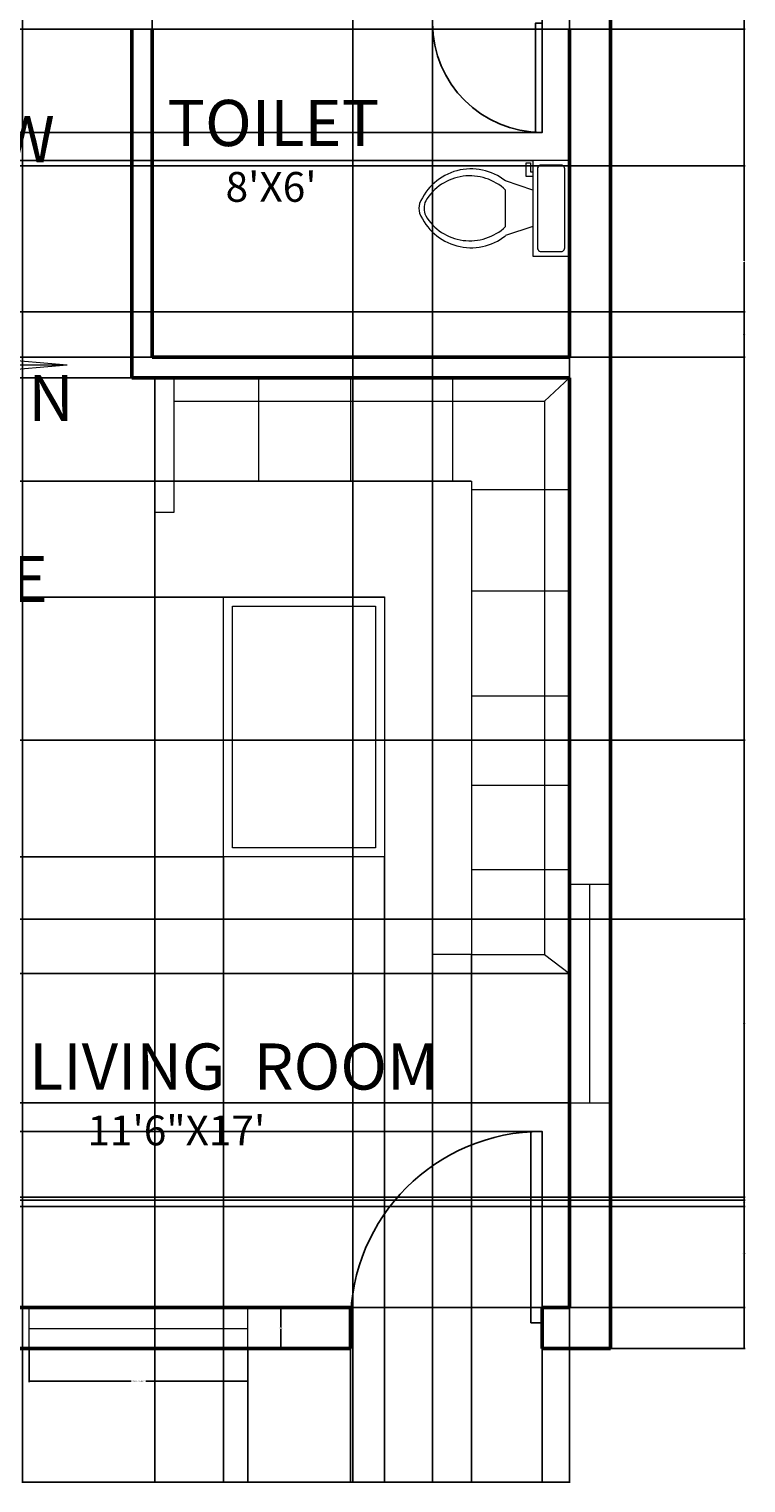
# Model space of a CAD drawing. Units: inches. Extents: x 19425 to 19848, y 45806 to 46417.
# Tile 4 of 5: x 19690 to 19848, y 45806 to 46125. Entities that reach past the tile are written whole.
import ezdxf

# ---------------------------------------------------------------- set-up
doc = ezdxf.new("R2010")
doc.units = ezdxf.units.IN
for name, color, linetype, lineweight in [('A-ANNO-DIMS', 2, 'Continuous', 18), ('A-ANNO-SYMB', 3, 'Continuous', 18), ('A-AREA-IDEN', 3, 'Continuous', 25), ('A-FLOR-FIXT', 2, 'Continuous', 20), ('door', 4, 'Continuous', 25), ('furniture', 2, 'Continuous', 18), ('wall', 6, 'Continuous', 50), ('window', 9, 'Continuous', 20)]:
    doc.layers.add(name, color=color, linetype=linetype, lineweight=lineweight)
doc.styles.get("Standard").update_dxf_attribs({"font": 'arial.ttf'})
doc.dimstyles.get("Standard").update_dxf_attribs({"dimtxt": 0.18, "dimasz": 0.18, "dimexe": 0.18, "dimexo": 0.0625, "dimgap": 0.09, "dimtad": 0, "dimtih": 1, "dimtoh": 1, "dimdec": 4, "dimzin": 0, "dimdsep": 46, "dimtxsty": 'Standard', "dimcen": 0.09, "dimadec": 0, "dimazin": 0, "dimtfac": 1, "dimtdec": 4, "dimtofl": 0, "dimtmove": 0, "dimatfit": 3, "dimfxl": 1, "dimtolj": 1, "dimtzin": 0, "dimarcsym": 0})

# ---------------------------------------------------------------- blocks, each defined once
blk = doc.blocks.new('*U2')
for p, q in [((0, 0), (0, -100)), ((750, 0), (750, -100))]:
    blk.add_line(p, q)
blk.add_lwpolyline([(0, 0), (0, 750), (43.75, 750), (43.75, 0)], close=True)
blk.add_arc((0, 0), 750, 0, 90)
blk = doc.blocks.new('Toilet - top')
for p, q in [((9.5, -6), (9.5, -2)), ((-10, -8.5), (-8, -8.5)), ((-10, -9.5), (-10, -8.5)), ((-7, -9.5), (-10, -9.5)), ((-8, -8.5), (-8, -8)), ((-7, -8), (-7, -9.5)), ((-4, -8), (-6, -14)), ((4, -8), (6, -14)), ((4, -14), (-4, -14))]:
    blk.add_line(p, q)
blk.add_lwpolyline([(10.5, -8), (10.5, 0), (-10.5, 0), (-10.5, -8)], close=True)
for points in [[(-9.5, -2), (-9.5, -6)], [(8.5, -1), (-8.5, -1)], [(-8.5, -7), (8.5, -7)]]:
    blk.add_lwpolyline(points)
for centre, radius, start, end in [((-8.62, -1.88), 0.884, 81.8699, 188.1301), ((8.62, -1.88), 0.884, 351.8699, 98.1301), ((-8.62, -6.12), 0.884, 171.8699, 278.1301), ((8.62, -6.12), 0.884, 261.8699, 8.1301), ((3.52, -21.58), 12.17, 141.4691, 247.9714), ((4.2, -21.82), 11.33, 136.3677, 238.9468), ((-3.52, -21.58), 12.17, 292.0284, 38.5307), ((-4.2, -21.82), 11.33, 301.053, 43.6321), ((0, -27.88), 4, 245.7318, 294.2682), ((0, -29), 4, 254.8605, 285.1395)]:
    blk.add_arc(centre, radius, start, end)
blk = doc.blocks.new('*U7')
at = {"layer": 'furniture'}
for p in [(-4.98, -28.71), (0, -23.73), (4.98, -28.71)]:
    blk.add_line(p, (0, 28.71), dxfattribs=at)
blk = doc.blocks.new('*U8')
at = {"layer": 'A-ANNO-SYMB', "transparency": 16777216}
blk.add_blockref('*U7', (19641.16, 46080.31), dxfattribs=at)
for p, rotation in [((19620.86, 46071.91), 45.00000000000001), ((19661.46, 46071.91), 315), ((19612.45, 46051.6), 90), ((19669.87, 46051.6), 270.0000000000001), ((19620.86, 46031.3), 135), ((19661.46, 46031.3), 225), ((19641.16, 46022.9), 180)]:
    blk.add_blockref('*U7', p, dxfattribs=dict(at, rotation=rotation))
blk = doc.blocks.new('WIN-48-CENTER-9')
for p, q in [((0, 48), (9, 48)), ((4.5, 0), (4.5, 48)), ((0, 0), (9, 0))]:
    blk.add_line(p, q)
blk = doc.blocks.new('WIN-48-OFFSET-9')
for p, q in [((0, 0), (0, 9)), ((48, 0), (48, 9)), ((48, 4.28), (0, 4.28))]:
    blk.add_line(p, q)
blk = doc.blocks.new('*D24')
at = {"layer": 'A-ANNO-DIMS', "color": 0, "lineweight": -2, "transparency": 16777216}
for p, q in [((19690.26, 45835.69), (19690.26, 45828.37)), ((19738.26, 45835.69), (19738.26, 45828.37)), ((19690.44, 45828.55), (19712.68, 45828.55)), ((19738.08, 45828.55), (19715.83, 45828.55))]:
    blk.add_line(p, q, dxfattribs=at)
at = {"layer": 'A-ANNO-DIMS', "color": 0, "transparency": 16777216}
for points in [[(19690.44, 45828.58), (19690.44, 45828.52), (19690.26, 45828.55)], [(19738.08, 45828.58), (19738.08, 45828.52), (19738.26, 45828.55)]]:
    blk.add_solid(points, dxfattribs=at)
at = {"layer": 'Defpoints', "color": 0, "transparency": 16777216}
for p in [(19690.26, 45835.75), (19738.26, 45835.75), (19738.26, 45828.55)]:
    blk.add_point(p, dxfattribs=at)
at = {"layer": 'A-ANNO-DIMS', "color": 0, "transparency": 16777216, "insert": (19714.26, 45828.55), "char_height": 0.18, "attachment_point": 5}
blk.add_mtext('\\A1;FRONT WINDOW 48 TYP.', dxfattribs=at)
blk = doc.blocks.new('*D25')
at = {"layer": 'A-ANNO-DIMS', "color": 0, "lineweight": -2, "transparency": 16777216}
for p, q in [((19738.32, 45844.75), (19745.64, 45844.75)), ((19745.46, 45844.57), (19745.46, 45840.44)), ((19745.46, 45835.93), (19745.46, 45840.07)), ((19738.32, 45835.75), (19745.64, 45835.75))]:
    blk.add_line(p, q, dxfattribs=at)
at = {"layer": 'A-ANNO-DIMS', "color": 0, "transparency": 16777216}
for points in [[(19745.43, 45844.57), (19745.49, 45844.57), (19745.46, 45844.75)], [(19745.43, 45835.93), (19745.49, 45835.93), (19745.46, 45835.75)]]:
    blk.add_solid(points, dxfattribs=at)
at = {"layer": 'Defpoints', "color": 0, "transparency": 16777216}
for p in [(19738.26, 45844.75), (19745.46, 45844.75), (19738.26, 45835.75)]:
    blk.add_point(p, dxfattribs=at)
at = {"layer": 'A-ANNO-DIMS', "color": 0, "transparency": 16777216, "insert": (19745.46, 45840.25), "char_height": 0.18, "attachment_point": 5}
blk.add_mtext('\\A1;9 TYP.', dxfattribs=at)
blk = doc.blocks.new('*D33')
at = {"layer": 'A-ANNO-DIMS', "color": 0, "lineweight": -2, "transparency": 16777216}
for p, q in [((19817.843662, 46312.754651), (19847.311162, 46312.754651)), ((19847.131162, 46312.574651), (19847.131162, 46074.434651)), ((19847.131162, 45835.934651), (19847.131162, 46074.074651)), ((19817.843662, 45835.754651), (19847.311162, 45835.754651))]:
    blk.add_line(p, q, dxfattribs=at)
at = {"layer": 'A-ANNO-DIMS', "color": 0, "transparency": 16777216}
for points in [[(19847.101162, 46312.574651), (19847.161162, 46312.574651), (19847.131162, 46312.754651)], [(19847.101162, 45835.934651), (19847.161162, 45835.934651), (19847.131162, 45835.754651)]]:
    blk.add_solid(points, dxfattribs=at)
at = {"layer": 'Defpoints', "color": 0, "transparency": 16777216}
for p in [(19817.781162, 46312.754651), (19847.131162, 46312.754651), (19817.781162, 45835.754651)]:
    blk.add_point(p, dxfattribs=at)
at = {"layer": 'A-ANNO-DIMS', "color": 0, "transparency": 16777216, "insert": (19847.131162, 46074.254651), "char_height": 0.18, "attachment_point": 5}
blk.add_mtext('\\A1;477', dxfattribs=at)
blk = doc.blocks.new('*D35')
at = {"layer": 'A-ANNO-DIMS', "color": 0, "lineweight": -2, "transparency": 16777216}
for p, q in [((19761.31, 46303.69), (19761.31, 45806.22)), ((19808.78, 46303.69), (19808.78, 45806.22)), ((19761.49, 45806.4), (19784.65, 45806.4)), ((19808.6, 45806.4), (19785.44, 45806.4))]:
    blk.add_line(p, q, dxfattribs=at)
at = {"layer": 'A-ANNO-DIMS', "color": 0, "transparency": 16777216}
for points in [[(19761.49, 45806.43), (19761.49, 45806.37), (19761.31, 45806.4)], [(19808.6, 45806.43), (19808.6, 45806.37), (19808.78, 45806.4)]]:
    blk.add_solid(points, dxfattribs=at)
at = {"layer": 'Defpoints', "color": 0, "transparency": 16777216}
for p in [(19761.31, 46303.75), (19808.78, 46303.75), (19808.78, 45806.4)]:
    blk.add_point(p, dxfattribs=at)
at = {"layer": 'A-ANNO-DIMS', "color": 0, "transparency": 16777216, "insert": (19785.04, 45806.4), "char_height": 0.18, "attachment_point": 5}
blk.add_mtext('\\A1;47.47', dxfattribs=at)
blk = doc.blocks.new('*D38')
at = {"layer": 'A-ANNO-DIMS', "color": 0, "lineweight": -2, "transparency": 16777216}
for p, q in [((19808.72, 45889.62), (19425.25, 45889.62)), ((19425.43, 45889.44), (19425.43, 45886.67)), ((19425.43, 45883.53), (19425.43, 45886.3)), ((19802.72, 45883.35), (19425.25, 45883.35))]:
    blk.add_line(p, q, dxfattribs=at)
at = {"layer": 'A-ANNO-DIMS', "color": 0, "transparency": 16777216}
for points in [[(19425.4, 45889.44), (19425.46, 45889.44), (19425.43, 45889.62)], [(19425.4, 45883.53), (19425.46, 45883.53), (19425.43, 45883.35)]]:
    blk.add_solid(points, dxfattribs=at)
at = {"layer": 'Defpoints', "color": 0, "transparency": 16777216}
for p in [(19425.43, 45889.62), (19808.78, 45889.62), (19802.78, 45883.35)]:
    blk.add_point(p, dxfattribs=at)
at = {"layer": 'A-ANNO-DIMS', "color": 0, "transparency": 16777216, "insert": (19425.43, 45886.49), "char_height": 0.18, "attachment_point": 5}
blk.add_mtext('\\A1;6.261', dxfattribs=at)
blk = doc.blocks.new('*D41')
at = {"layer": 'A-ANNO-DIMS', "color": 0, "lineweight": -2, "transparency": 16777216}
for p, q in [((19738.26, 45835.69), (19738.26, 45806.22)), ((19760.78, 45835.69), (19760.78, 45806.22)), ((19738.44, 45806.4), (19749.05, 45806.4)), ((19760.6, 45806.4), (19749.98, 45806.4))]:
    blk.add_line(p, q, dxfattribs=at)
at = {"layer": 'A-ANNO-DIMS', "color": 0, "transparency": 16777216}
for points in [[(19738.44, 45806.43), (19738.44, 45806.37), (19738.26, 45806.4)], [(19760.6, 45806.43), (19760.6, 45806.37), (19760.78, 45806.4)]]:
    blk.add_solid(points, dxfattribs=at)
at = {"layer": 'Defpoints', "color": 0, "transparency": 16777216}
for p in [(19738.26, 45835.75), (19760.78, 45835.75), (19760.78, 45806.4)]:
    blk.add_point(p, dxfattribs=at)
at = {"layer": 'A-ANNO-DIMS', "color": 0, "transparency": 16777216, "insert": (19749.52, 45806.4), "char_height": 0.18, "attachment_point": 5}
blk.add_mtext('\\A1;22.526', dxfattribs=at)
blk = doc.blocks.new('*D42')
at = {"layer": 'A-ANNO-DIMS', "color": 0, "lineweight": -2, "transparency": 16777216}
for p, q in [((19760.78, 45835.69), (19760.78, 45806.22)), ((19802.78, 45835.69), (19802.78, 45806.22)), ((19760.96, 45806.4), (19781.56, 45806.4)), ((19802.6, 45806.4), (19782, 45806.4))]:
    blk.add_line(p, q, dxfattribs=at)
at = {"layer": 'A-ANNO-DIMS', "color": 0, "transparency": 16777216}
for points in [[(19760.96, 45806.43), (19760.96, 45806.37), (19760.78, 45806.4)], [(19802.6, 45806.43), (19802.6, 45806.37), (19802.78, 45806.4)]]:
    blk.add_solid(points, dxfattribs=at)
at = {"layer": 'Defpoints', "color": 0, "transparency": 16777216}
for p in [(19760.78, 45835.75), (19802.78, 45835.75), (19802.78, 45806.4)]:
    blk.add_point(p, dxfattribs=at)
at = {"layer": 'A-ANNO-DIMS', "color": 0, "transparency": 16777216, "insert": (19781.78, 45806.4), "char_height": 0.18, "attachment_point": 5}
blk.add_mtext('\\A1;42', dxfattribs=at)
blk = doc.blocks.new('*D50')
at = {"layer": 'A-ANNO-DIMS', "color": 0, "lineweight": -2, "transparency": 16777216}
for p, q in [((19625.38, 45929.95), (19847.31, 45929.95)), ((19847.13, 45929.77), (19847.13, 45899.3)), ((19847.13, 45868.46), (19847.13, 45898.93)), ((19625.38, 45868.28), (19847.31, 45868.28))]:
    blk.add_line(p, q, dxfattribs=at)
at = {"layer": 'A-ANNO-DIMS', "color": 0, "transparency": 16777216}
for points in [[(19847.1, 45929.77), (19847.16, 45929.77), (19847.13, 45929.95)], [(19847.1, 45868.46), (19847.16, 45868.46), (19847.13, 45868.28)]]:
    blk.add_solid(points, dxfattribs=at)
at = {"layer": 'Defpoints', "color": 0, "transparency": 16777216}
for p in [(19625.31, 45929.95), (19847.13, 45929.95), (19625.31, 45868.28)]:
    blk.add_point(p, dxfattribs=at)
at = {"layer": 'A-ANNO-DIMS', "color": 0, "transparency": 16777216, "insert": (19847.13, 45899.11), "char_height": 0.18, "attachment_point": 5}
blk.add_mtext('\\A1;61.67', dxfattribs=at)
blk = doc.blocks.new('*D51')
at = {"layer": 'A-ANNO-DIMS', "color": 0, "lineweight": -2, "transparency": 16777216}
for p, q in [((19732.87, 45943.55), (19732.87, 45806.22)), ((19768.22, 45943.55), (19768.22, 45806.22)), ((19733.05, 45806.4), (19750.15, 45806.4)), ((19768.04, 45806.4), (19750.94, 45806.4))]:
    blk.add_line(p, q, dxfattribs=at)
at = {"layer": 'A-ANNO-DIMS', "color": 0, "transparency": 16777216}
for points in [[(19733.05, 45806.43), (19733.05, 45806.37), (19732.87, 45806.4)], [(19768.04, 45806.43), (19768.04, 45806.37), (19768.22, 45806.4)]]:
    blk.add_solid(points, dxfattribs=at)
at = {"layer": 'Defpoints', "color": 0, "transparency": 16777216}
for p in [(19732.87, 45943.61), (19768.22, 45943.61), (19768.22, 45806.4)]:
    blk.add_point(p, dxfattribs=at)
at = {"layer": 'A-ANNO-DIMS', "color": 0, "transparency": 16777216, "insert": (19750.55, 45806.4), "char_height": 0.18, "attachment_point": 5}
blk.add_mtext('\\A1;35.34', dxfattribs=at)
blk = doc.blocks.new('*D52')
at = {"layer": 'A-ANNO-DIMS', "color": 0, "lineweight": -2, "transparency": 16777216}
for p, q in [((19732.81, 46000.63), (19425.25, 46000.63)), ((19425.43, 46000.45), (19425.43, 45972.3)), ((19425.43, 45943.79), (19425.43, 45971.94)), ((19732.81, 45943.61), (19425.25, 45943.61))]:
    blk.add_line(p, q, dxfattribs=at)
at = {"layer": 'A-ANNO-DIMS', "color": 0, "transparency": 16777216}
for points in [[(19425.4, 46000.45), (19425.46, 46000.45), (19425.43, 46000.63)], [(19425.4, 45943.79), (19425.46, 45943.79), (19425.43, 45943.61)]]:
    blk.add_solid(points, dxfattribs=at)
at = {"layer": 'Defpoints', "color": 0, "transparency": 16777216}
for p in [(19425.43, 46000.63), (19732.87, 46000.63), (19732.87, 45943.61)]:
    blk.add_point(p, dxfattribs=at)
at = {"layer": 'A-ANNO-DIMS', "color": 0, "transparency": 16777216, "insert": (19425.43, 45972.12), "char_height": 0.18, "attachment_point": 5}
blk.add_mtext('\\A1;57.02', dxfattribs=at)
blk = doc.blocks.new('*D53')
at = {"layer": 'A-ANNO-DIMS', "color": 0, "lineweight": -2, "transparency": 16777216}
for p, q in [((19717.85, 46048.69), (19717.85, 45806.22)), ((19808.78, 46048.69), (19808.78, 45806.22)), ((19718.03, 45806.4), (19762.92, 45806.4)), ((19808.6, 45806.4), (19763.71, 45806.4))]:
    blk.add_line(p, q, dxfattribs=at)
at = {"layer": 'A-ANNO-DIMS', "color": 0, "transparency": 16777216}
for points in [[(19718.03, 45806.43), (19718.03, 45806.37), (19717.85, 45806.4)], [(19808.6, 45806.43), (19808.6, 45806.37), (19808.78, 45806.4)]]:
    blk.add_solid(points, dxfattribs=at)
at = {"layer": 'Defpoints', "color": 0, "transparency": 16777216}
for p in [(19717.85, 46048.75), (19808.78, 46048.75), (19808.78, 45806.4)]:
    blk.add_point(p, dxfattribs=at)
at = {"layer": 'A-ANNO-DIMS', "color": 0, "transparency": 16777216, "insert": (19763.32, 45806.4), "char_height": 0.18, "attachment_point": 5}
blk.add_mtext('\\A1;90.93', dxfattribs=at)
blk = doc.blocks.new('*D54')
at = {"layer": 'A-ANNO-DIMS', "color": 0, "lineweight": -2, "transparency": 16777216}
for p, q in [((19808.72, 46048.75), (19425.25, 46048.75)), ((19425.43, 46048.57), (19425.43, 45983.58)), ((19425.43, 45918.22), (19425.43, 45983.22)), ((19808.72, 45918.04), (19425.25, 45918.04))]:
    blk.add_line(p, q, dxfattribs=at)
at = {"layer": 'A-ANNO-DIMS', "color": 0, "transparency": 16777216}
for points in [[(19425.4, 46048.57), (19425.46, 46048.57), (19425.43, 46048.75)], [(19425.4, 45918.22), (19425.46, 45918.22), (19425.43, 45918.04)]]:
    blk.add_solid(points, dxfattribs=at)
at = {"layer": 'Defpoints', "color": 0, "transparency": 16777216}
for p in [(19425.43, 46048.75), (19808.78, 46048.75), (19808.78, 45918.04)]:
    blk.add_point(p, dxfattribs=at)
at = {"layer": 'A-ANNO-DIMS', "color": 0, "transparency": 16777216, "insert": (19425.43, 45983.4), "char_height": 0.18, "attachment_point": 5}
blk.add_mtext('\\A1;130.7', dxfattribs=at)
blk = doc.blocks.new('*D55')
at = {"layer": 'A-ANNO-DIMS', "color": 0, "lineweight": -2, "transparency": 16777216}
for p, q in [((19717.28, 46053.32), (19717.28, 46342.28)), ((19717.46, 46342.1), (19762.71, 46342.1)), ((19808.6, 46342.1), (19763.36, 46342.1)), ((19808.78, 46053.32), (19808.78, 46342.28))]:
    blk.add_line(p, q, dxfattribs=at)
at = {"layer": 'A-ANNO-DIMS', "color": 0, "transparency": 16777216}
for points in [[(19717.46, 46342.13), (19717.46, 46342.07), (19717.28, 46342.1)], [(19808.6, 46342.13), (19808.6, 46342.07), (19808.78, 46342.1)]]:
    blk.add_solid(points, dxfattribs=at)
at = {"layer": 'Defpoints', "color": 0, "transparency": 16777216}
for p in [(19808.78, 46342.1), (19717.28, 46053.25), (19808.78, 46053.25)]:
    blk.add_point(p, dxfattribs=at)
at = {"layer": 'A-ANNO-DIMS', "color": 0, "transparency": 16777216, "insert": (19763.03, 46342.1), "char_height": 0.18, "attachment_point": 5}
blk.add_mtext('\\A1;91.5', dxfattribs=at)
blk = doc.blocks.new('*D57')
at = {"layer": 'A-ANNO-DIMS', "color": 0, "lineweight": -2, "transparency": 16777216}
for p, q in [((19625.38, 45868.28), (19847.31, 45868.28)), ((19847.13, 45868.1), (19847.13, 45856.7)), ((19847.13, 45844.93), (19847.13, 45856.33)), ((19638.06, 45844.75), (19847.31, 45844.75))]:
    blk.add_line(p, q, dxfattribs=at)
at = {"layer": 'A-ANNO-DIMS', "color": 0, "transparency": 16777216}
for points in [[(19847.1, 45868.1), (19847.16, 45868.1), (19847.13, 45868.28)], [(19847.1, 45844.93), (19847.16, 45844.93), (19847.13, 45844.75)]]:
    blk.add_solid(points, dxfattribs=at)
at = {"layer": 'Defpoints', "color": 0, "transparency": 16777216}
for p in [(19625.31, 45868.28), (19638, 45844.75), (19847.13, 45844.75)]:
    blk.add_point(p, dxfattribs=at)
at = {"layer": 'A-ANNO-DIMS', "color": 0, "transparency": 16777216, "insert": (19847.13, 45856.52), "char_height": 0.18, "attachment_point": 5}
blk.add_mtext('\\A1;23.524', dxfattribs=at)
blk = doc.blocks.new('*D66')
at = {"layer": 'A-ANNO-DIMS', "color": 0, "lineweight": -2, "transparency": 16777216}
for p, q in [((19559.84, 46063.22), (19847.31, 46063.22)), ((19847.13, 46063.04), (19847.13, 46058.42)), ((19847.13, 46053.43), (19847.13, 46058.06)), ((19559.84, 46053.25), (19847.31, 46053.25))]:
    blk.add_line(p, q, dxfattribs=at)
at = {"layer": 'A-ANNO-DIMS', "color": 0, "transparency": 16777216}
for points in [[(19847.1, 46063.04), (19847.16, 46063.04), (19847.13, 46063.22)], [(19847.1, 46053.43), (19847.16, 46053.43), (19847.13, 46053.25)]]:
    blk.add_solid(points, dxfattribs=at)
at = {"layer": 'Defpoints', "color": 0, "transparency": 16777216}
for p in [(19559.78, 46063.22), (19847.13, 46063.22), (19559.78, 46053.25)]:
    blk.add_point(p, dxfattribs=at)
at = {"layer": 'A-ANNO-DIMS', "color": 0, "transparency": 16777216, "insert": (19847.13, 46058.24), "char_height": 0.18, "attachment_point": 5}
blk.add_mtext('\\A1;9.967', dxfattribs=at)
blk = doc.blocks.new('*D67')
at = {"layer": 'A-ANNO-DIMS', "color": 0, "lineweight": -2, "transparency": 16777216}
for p, q in [((19564.34, 46125.25), (19847.31, 46125.25)), ((19847.13, 46125.07), (19847.13, 46110.44)), ((19847.13, 46095.43), (19847.13, 46110.07)), ((19564.34, 46095.25), (19847.31, 46095.25))]:
    blk.add_line(p, q, dxfattribs=at)
at = {"layer": 'A-ANNO-DIMS', "color": 0, "transparency": 16777216}
for points in [[(19847.1, 46125.07), (19847.16, 46125.07), (19847.13, 46125.25)], [(19847.1, 46095.43), (19847.16, 46095.43), (19847.13, 46095.25)]]:
    blk.add_solid(points, dxfattribs=at)
at = {"layer": 'Defpoints', "color": 0, "transparency": 16777216}
for p in [(19564.28, 46125.25), (19847.13, 46125.25), (19564.28, 46095.25)]:
    blk.add_point(p, dxfattribs=at)
at = {"layer": 'A-ANNO-DIMS', "color": 0, "transparency": 16777216, "insert": (19847.13, 46110.25), "char_height": 0.18, "attachment_point": 5}
blk.add_mtext('\\A1;30', dxfattribs=at)
blk = doc.blocks.new('*D68')
at = {"layer": 'A-ANNO-DIMS', "color": 0, "lineweight": -2, "transparency": 16777216}
for p, q in [((19768.22, 45943.55), (19768.22, 45806.22)), ((19787.29, 45922.11), (19787.29, 45806.22)), ((19768.4, 45806.4), (19777.37, 45806.4)), ((19787.11, 45806.4), (19778.14, 45806.4))]:
    blk.add_line(p, q, dxfattribs=at)
at = {"layer": 'A-ANNO-DIMS', "color": 0, "transparency": 16777216}
for points in [[(19768.4, 45806.43), (19768.4, 45806.37), (19768.22, 45806.4)], [(19787.11, 45806.43), (19787.11, 45806.37), (19787.29, 45806.4)]]:
    blk.add_solid(points, dxfattribs=at)
at = {"layer": 'Defpoints', "color": 0, "transparency": 16777216}
for p in [(19768.22, 45943.61), (19787.29, 45922.17), (19787.29, 45806.4)]:
    blk.add_point(p, dxfattribs=at)
at = {"layer": 'A-ANNO-DIMS', "color": 0, "transparency": 16777216, "insert": (19777.75, 45806.4), "char_height": 0.18, "attachment_point": 5}
blk.add_mtext('\\A1;19.07', dxfattribs=at)
blk = doc.blocks.new('*D69')
at = {"layer": 'A-ANNO-DIMS', "color": 0, "lineweight": -2, "transparency": 16777216}
for p, q in [((19787.22, 46026.07), (19425.25, 46026.07)), ((19425.43, 46025.89), (19425.43, 46013.53)), ((19425.43, 46000.81), (19425.43, 46013.17)), ((19768.15, 46000.63), (19425.25, 46000.63))]:
    blk.add_line(p, q, dxfattribs=at)
at = {"layer": 'A-ANNO-DIMS', "color": 0, "transparency": 16777216}
for points in [[(19425.4, 46025.89), (19425.46, 46025.89), (19425.43, 46026.07)], [(19425.4, 46000.81), (19425.46, 46000.81), (19425.43, 46000.63)]]:
    blk.add_solid(points, dxfattribs=at)
at = {"layer": 'Defpoints', "color": 0, "transparency": 16777216}
for p in [(19425.43, 46026.07), (19787.29, 46026.07), (19768.22, 46000.63)]:
    blk.add_point(p, dxfattribs=at)
at = {"layer": 'A-ANNO-DIMS', "color": 0, "transparency": 16777216, "insert": (19425.43, 46013.35), "char_height": 0.18, "attachment_point": 5}
blk.add_mtext('\\A1;25.44', dxfattribs=at)
blk = doc.blocks.new('*D70')
at = {"layer": 'A-ANNO-DIMS', "color": 0, "lineweight": -2, "transparency": 16777216}
for p, q in [((19666.34, 45969.25), (19847.31, 45969.25)), ((19847.13, 45969.07), (19847.13, 45907.19)), ((19847.13, 45844.93), (19847.13, 45906.82)), ((19666.34, 45844.75), (19847.31, 45844.75))]:
    blk.add_line(p, q, dxfattribs=at)
at = {"layer": 'A-ANNO-DIMS', "color": 0, "transparency": 16777216}
for points in [[(19847.1, 45969.07), (19847.16, 45969.07), (19847.13, 45969.25)], [(19847.1, 45844.93), (19847.16, 45844.93), (19847.13, 45844.75)]]:
    blk.add_solid(points, dxfattribs=at)
at = {"layer": 'Defpoints', "color": 0, "transparency": 16777216}
for p in [(19666.28, 45969.25), (19847.13, 45969.25), (19666.28, 45844.75)]:
    blk.add_point(p, dxfattribs=at)
at = {"layer": 'A-ANNO-DIMS', "color": 0, "transparency": 16777216, "insert": (19847.13, 45907), "char_height": 0.18, "attachment_point": 5}
blk.add_mtext('\\A1;124.5', dxfattribs=at)
blk = doc.blocks.new('*D74')
at = {"layer": 'A-ANNO-DIMS', "color": 0, "lineweight": -2, "transparency": 16777216}
for p, q in [((19688.78, 46129.69), (19688.78, 45806.22)), ((19778.78, 46129.69), (19778.78, 45806.22)), ((19688.96, 45806.4), (19733.56, 45806.4)), ((19778.6, 45806.4), (19734, 45806.4))]:
    blk.add_line(p, q, dxfattribs=at)
at = {"layer": 'A-ANNO-DIMS', "color": 0, "transparency": 16777216}
for points in [[(19688.96, 45806.43), (19688.96, 45806.37), (19688.78, 45806.4)], [(19778.6, 45806.43), (19778.6, 45806.37), (19778.78, 45806.4)]]:
    blk.add_solid(points, dxfattribs=at)
at = {"layer": 'Defpoints', "color": 0, "transparency": 16777216}
for p in [(19688.78, 46129.75), (19778.78, 46129.75), (19778.78, 45806.4)]:
    blk.add_point(p, dxfattribs=at)
at = {"layer": 'A-ANNO-DIMS', "color": 0, "transparency": 16777216, "insert": (19733.78, 45806.4), "char_height": 0.18, "attachment_point": 5}
blk.add_mtext('\\A1;90', dxfattribs=at)
blk = doc.blocks.new('*D75')
at = {"layer": 'A-ANNO-DIMS', "color": 0, "lineweight": -2, "transparency": 16777216}
for p, q in [((19802.72, 46102.55), (19425.25, 46102.55)), ((19425.43, 46102.37), (19425.43, 46099.67)), ((19425.43, 46096.6), (19425.43, 46099.31)), ((19800.72, 46096.42), (19425.25, 46096.42))]:
    blk.add_line(p, q, dxfattribs=at)
at = {"layer": 'A-ANNO-DIMS', "color": 0, "transparency": 16777216}
for points in [[(19425.4, 46102.37), (19425.46, 46102.37), (19425.43, 46102.55)], [(19425.4, 46096.6), (19425.46, 46096.6), (19425.43, 46096.42)]]:
    blk.add_solid(points, dxfattribs=at)
at = {"layer": 'Defpoints', "color": 0, "transparency": 16777216}
for p in [(19802.78, 46102.55), (19425.43, 46096.42), (19800.78, 46096.42)]:
    blk.add_point(p, dxfattribs=at)
at = {"layer": 'A-ANNO-DIMS', "color": 0, "transparency": 16777216, "insert": (19425.43, 46099.49), "char_height": 0.18, "attachment_point": 5}
blk.add_mtext('\\A1;6.134', dxfattribs=at)
blk = doc.blocks.new('*D76')
at = {"layer": 'A-ANNO-DIMS', "color": 0, "lineweight": -2, "transparency": 16777216}
for p, q in [((19463.84, 45868.92), (19847.31, 45868.92)), ((19847.13, 45868.74), (19847.13, 45868.09)), ((19847.13, 45867.09), (19847.13, 45867.73)), ((19465.78, 45866.91), (19847.31, 45866.91))]:
    blk.add_line(p, q, dxfattribs=at)
at = {"layer": 'A-ANNO-DIMS', "color": 0, "transparency": 16777216}
for points in [[(19847.1, 45868.74), (19847.16, 45868.74), (19847.13, 45868.92)], [(19847.1, 45867.09), (19847.16, 45867.09), (19847.13, 45866.91)]]:
    blk.add_solid(points, dxfattribs=at)
at = {"layer": 'Defpoints', "color": 0, "transparency": 16777216}
for p in [(19463.78, 45868.92), (19465.72, 45866.91), (19847.13, 45866.91)]:
    blk.add_point(p, dxfattribs=at)
at = {"layer": 'A-ANNO-DIMS', "color": 0, "transparency": 16777216, "insert": (19847.13, 45867.91), "char_height": 0.18, "attachment_point": 5}
blk.add_mtext('\\A1;2.01', dxfattribs=at)

msp = doc.modelspace()

# ---------------------------------------------------------------- linework, layer by layer
at = {"layer": 'furniture'}
for p, q in [((19717.8513, 46019.1956), (19717.8513, 46048.7547)), ((19722.0064, 46048.7547), (19722.0064, 46026.0705)), ((19740.5598, 46048.7547), (19740.5598, 46026.0705)), ((19760.7812, 46048.7547), (19760.7812, 46026.0705)), ((19783.2432, 46026.0705), (19783.2432, 46048.7547)), ((19803.293, 46043.6348), (19808.7812, 46048.7547)), ((19722.0064, 46043.6348), (19803.293, 46043.6348)), ((19803.293, 46043.6348), (19803.293, 45922.1684)), ((19722.0064, 46026.0705), (19787.2853, 46026.0705)), ((19722.0064, 46026.0705), (19722.0064, 46019.1956)), ((19787.2853, 46026.0705), (19787.2853, 45922.1684)), ((19787.2853, 46024.2366), (19808.7812, 46024.2366)), ((19722.0064, 46019.1956), (19717.8513, 46019.1956)), ((19787.2853, 46002.0174), (19808.7812, 46002.0174)), ((19787.2853, 45978.9638), (19808.7812, 45978.9638)), ((19787.2853, 45959.3603), (19808.7812, 45959.3603)), ((19787.2853, 45940.8612), (19808.7812, 45940.8612)), ((19787.2853, 45922.1684), (19778.7403, 45922.1684)), ((19778.7403, 45922.1684), (19778.7403, 45918.0438)), ((19787.2853, 45922.1684), (19803.293, 45922.1684)), ((19803.293, 45922.1684), (19808.7812, 45918.0438)), ((19778.7403, 45918.0438), (19808.7812, 45918.0438))]:
    msp.add_line(p, q, dxfattribs=at)
for points in [[(19732.8741, 46000.631), (19768.2171, 46000.631), (19768.2171, 45943.6092), (19732.8741, 45943.6092)], [(19734.8741, 45998.631), (19766.2171, 45998.631), (19766.2171, 45945.6092), (19734.8741, 45945.6092)]]:
    msp.add_lwpolyline(points, close=True, dxfattribs=at)
at = {"layer": 'wall'}
for p, q in [((19817.7812, 46312.7547), (19817.7812, 45835.7547)), ((19712.7812, 46125.2547), (19712.7812, 46048.7547)), ((19717.2812, 46125.2547), (19717.2812, 46053.2547)), ((19808.7812, 46125.2547), (19808.7812, 46053.2547)), ((19717.2812, 46053.2547), (19808.7812, 46053.2547)), ((19712.7812, 46048.7547), (19808.7812, 46048.7547)), ((19808.7812, 46048.7547), (19808.7812, 45969.2547)), ((19808.7812, 46048.7547), (19808.7812, 45844.7547)), ((19670.7812, 45844.7547), (19760.7812, 45844.7547)), ((19760.7812, 45844.7547), (19760.7812, 45835.7547)), ((19802.7812, 45844.7547), (19802.7812, 45835.7547)), ((19802.7812, 45844.7547), (19808.7812, 45844.7547)), ((19454.7812, 45835.7547), (19760.7812, 45835.7547)), ((19802.7812, 45835.7547), (19817.7812, 45835.7547))]:
    msp.add_line(p, q, dxfattribs=at)

# ---------------------------------------------------------------- block references
at = {"layer": 'A-ANNO-SYMB'}
msp.add_blockref('*U8', (0, 0), dxfattribs=at)
at = {"layer": 'A-FLOR-FIXT', "rotation": 270}
msp.add_blockref('Toilet - top', (19808.7812, 46085.9211), dxfattribs=at)
at = {"layer": 'door', "xscale": 0.0320000000000009, "yscale": 0.0320000000000009, "zscale": 0.0320000000000009, "rotation": 180}
msp.add_blockref('*U2', (19802.7812, 46126.5547), dxfattribs=at)
at = {"layer": 'door', "xscale": -0.0560000000000015, "yscale": 0.0560000000000015, "zscale": 0.0560000000000015}
msp.add_blockref('*U2', (19802.7812, 45841.3547), dxfattribs=at)
at = {"layer": 'window'}
for name, p in [('WIN-48-CENTER-9', (19808.7812, 45889.6159)), ('WIN-48-OFFSET-9', (19690.2556, 45835.7547))]:
    msp.add_blockref(name, p, dxfattribs=at)

# ---------------------------------------------------------------- texts
at = {"layer": 'A-ANNO-SYMB'}
for s, height, p in [('NW', 10.12861, (19673.7783, 46096.0476)), ('N', 10.1286, (19690.0685, 46039.2189)), ('NE', 10.12861, (19676.2165, 45999.5028))]:
    msp.add_text(s, height=height, dxfattribs=at).set_placement(p)
at = {"layer": 'A-AREA-IDEN'}
for s, height, p in [('TOILET', 10.12861, (19720.5798, 46099.5832)), ("8'X6'", 6.53608, (19733.3601, 46087.3572)), ('LIVING  ROOM', 10.128615, (19690.2571, 45892.5309)), ('11\'6"X17\'', 6.53608, (19703.0374, 45880.3049))]:
    msp.add_text(s, height=height, dxfattribs=at).set_placement(p)

# ---------------------------------------------------------------- dimensions: what is measured, and where the dimension line sits
at = {"layer": 'A-ANNO-DIMS'}
for base, p1, p2, override, picture, middle in [((19808.7812, 46342.1047), (19717.2812, 46053.2547), (19808.7812, 46053.2547), {"dimdec": 1, "dimlfac": 1, "dimrnd": 0, "dimzin": 0, "dimdsep": 46, "dimlunit": 2}, '*D55', (19763.0312, 46342.1047)), ((19808.7812, 45806.4047), (19761.3082, 46303.7547), (19808.7812, 46303.7547), {"dimdec": 2, "dimlfac": 1, "dimrnd": 0, "dimzin": 0, "dimdsep": 46, "dimlunit": 2}, '*D35', (19785.0447, 45806.4047)), ((19778.7812, 45806.4047), (19688.7812, 46129.7547), (19778.7812, 46129.7547), {"dimdec": 0, "dimlfac": 1, "dimrnd": 0, "dimzin": 0, "dimdsep": 46, "dimlunit": 2}, '*D74', (19733.7812, 45806.4047)), ((19808.7812, 45806.4047), (19717.8513, 46048.7547), (19808.7812, 46048.7547), {"dimdec": 2, "dimlfac": 1, "dimrnd": 0, "dimzin": 0, "dimdsep": 46, "dimlunit": 2}, '*D53', (19763.3162, 45806.4047)), ((19768.2171, 45806.4047), (19732.8741, 45943.6092), (19768.2171, 45943.6092), {"dimdec": 2, "dimlfac": 1, "dimrnd": 0, "dimzin": 0, "dimdsep": 46, "dimlunit": 2}, '*D51', (19750.5456, 45806.4047)), ((19787.2853, 45806.4047), (19768.2171, 45943.6092), (19787.2853, 45922.1684), {"dimdec": 2, "dimlfac": 1, "dimrnd": 0, "dimzin": 0, "dimdsep": 46, "dimlunit": 2}, '*D68', (19777.7512, 45806.4047)), ((19760.7812, 45806.4047), (19738.2556, 45835.7547), (19760.7812, 45835.7547), {"dimdec": 3, "dimlfac": 1, "dimrnd": 0, "dimzin": 0, "dimdsep": 46, "dimlunit": 2}, '*D41', (19749.5184, 45806.4047)), ((19802.7812, 45806.4047), (19760.7812, 45835.7547), (19802.7812, 45835.7547), {"dimdec": 0, "dimlfac": 1, "dimrnd": 0, "dimzin": 0, "dimdsep": 46, "dimlunit": 2}, '*D42', (19781.7812, 45806.4047))]:
    dim = msp.add_linear_dim(base=base, p1=p1, p2=p2, dimstyle='Standard', override=override, dxfattribs=at)
    dim.commit()
    dim.dimension.update_dxf_attribs({"geometry": picture, "text_midpoint": middle})
for base, p1, p2, override, picture, middle in [((19847.1312, 46312.7547), (19817.7812, 45835.7547), (19817.7812, 46312.7547), {"dimdec": 0, "dimlfac": 1, "dimrnd": 0, "dimzin": 0, "dimdsep": 46, "dimlunit": 2}, '*D33', (19847.1312, 46074.2547)), ((19847.1312, 46125.2547), (19564.2812, 46095.2547), (19564.2812, 46125.2547), {"dimdec": 0, "dimlfac": 1, "dimrnd": 0, "dimzin": 0, "dimdsep": 46, "dimlunit": 2}, '*D67', (19847.1312, 46110.2547)), ((19425.4312, 46096.4211), (19802.7812, 46102.5547), (19800.7812, 46096.4211), {"dimdec": 3, "dimlfac": 1, "dimrnd": 0, "dimzin": 0, "dimdsep": 46, "dimlunit": 2}, '*D75', (19425.4312, 46099.4879)), ((19847.1312, 46063.2218), (19559.7812, 46053.2547), (19559.7812, 46063.2218), {"dimdec": 3, "dimlfac": 1, "dimrnd": 0, "dimzin": 0, "dimdsep": 46, "dimlunit": 2}, '*D66', (19847.1312, 46058.2382)), ((19425.4312, 46048.7547), (19808.7812, 45918.0438), (19808.7812, 46048.7547), {"dimdec": 1, "dimlfac": 1, "dimrnd": 0, "dimzin": 0, "dimdsep": 46, "dimlunit": 2}, '*D54', (19425.4312, 45983.3992)), ((19425.4312, 46026.0705), (19768.2171, 46000.631), (19787.2853, 46026.0705), {"dimdec": 2, "dimlfac": 1, "dimrnd": 0, "dimzin": 0, "dimdsep": 46, "dimlunit": 2}, '*D69', (19425.4312, 46013.3508)), ((19425.4312, 46000.631), (19732.8741, 45943.6092), (19732.8741, 46000.631), {"dimdec": 2, "dimlfac": 1, "dimrnd": 0, "dimzin": 0, "dimdsep": 46, "dimlunit": 2}, '*D52', (19425.4312, 45972.1201)), ((19847.1312, 45969.2547), (19666.2812, 45844.7547), (19666.2812, 45969.2547), {"dimdec": 1, "dimlfac": 1, "dimrnd": 0, "dimzin": 0, "dimdsep": 46, "dimlunit": 2}, '*D70', (19847.1312, 45907.0047)), ((19847.1312, 45929.95), (19625.3129, 45868.2782), (19625.3129, 45929.95), {"dimdec": 2, "dimlfac": 1, "dimrnd": 0, "dimzin": 0, "dimdsep": 46, "dimlunit": 2}, '*D50', (19847.1312, 45899.1141)), ((19425.4312, 45889.6159), (19802.7812, 45883.3547), (19808.7812, 45889.6159), {"dimdec": 3, "dimlfac": 1, "dimrnd": 0, "dimzin": 0, "dimdsep": 46, "dimlunit": 2}, '*D38', (19425.4312, 45886.4853)), ((19847.1312, 45866.9088), (19463.7812, 45868.9163), (19465.7192, 45866.9088), {"dimdec": 2, "dimlfac": 1, "dimrnd": 0, "dimzin": 0, "dimdsep": 46, "dimlunit": 2}, '*D76', (19847.1312, 45867.9126)), ((19847.13116, 45844.75465), (19625.31287, 45868.27825), (19637.99712, 45844.75465), {"dimdec": 3, "dimlfac": 1, "dimrnd": 0, "dimzin": 0, "dimdsep": 46, "dimlunit": 2}, '*D57', (19847.13116, 45856.51645))]:
    dim = msp.add_linear_dim(base=base, p1=p1, p2=p2, angle=90, dimstyle='Standard', override=override, dxfattribs=at)
    dim.commit()
    dim.dimension.update_dxf_attribs({"geometry": picture, "text_midpoint": middle})
dim = msp.add_linear_dim(base=(19745.4556, 45844.7547), p1=(19738.2556, 45835.7547), p2=(19738.2556, 45844.7547), angle=90, text='<> TYP.', dimstyle='Standard', override={"dimdec": 0, "dimlfac": 1, "dimrnd": 0, "dimzin": 0, "dimdsep": 46, "dimlunit": 2}, dxfattribs=at)
dim.commit()
dim.dimension.update_dxf_attribs({"geometry": '*D25', "text_midpoint": (19745.4556, 45840.2547)})
dim = msp.add_linear_dim(base=(19738.2556, 45828.5547), p1=(19690.2556, 45835.7547), p2=(19738.2556, 45835.7547), text='FRONT WINDOW <> TYP.', dimstyle='Standard', override={"dimdec": 0, "dimlfac": 1, "dimrnd": 0, "dimzin": 0, "dimdsep": 46, "dimlunit": 2}, dxfattribs=at)
dim.commit()
dim.dimension.update_dxf_attribs({"geometry": '*D24', "text_midpoint": (19714.2556, 45828.5547)})

doc.saveas('drawing.dxf')
